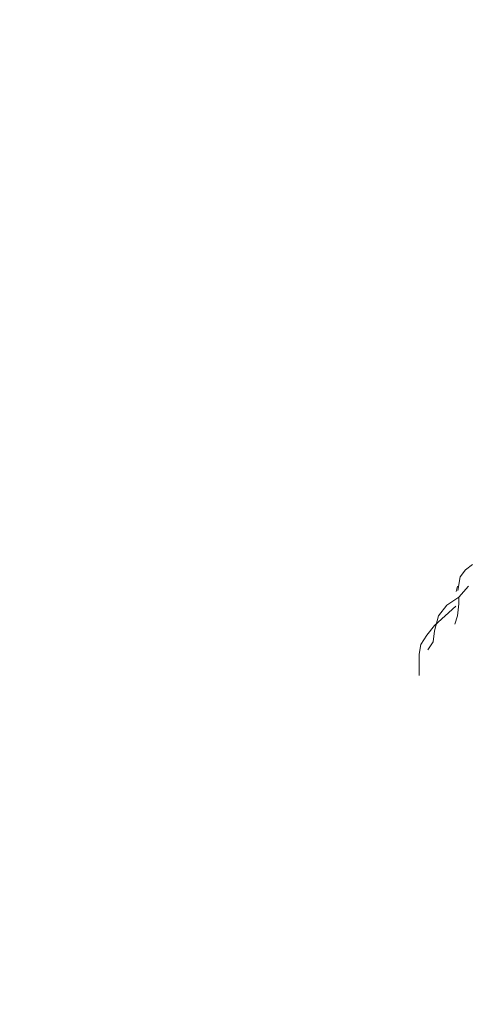
# Model space of a CAD drawing. Units: millimetres. Extents: x 595116 to 630915, y 909473 to 920225.
# Tile 81 of 134: x 629702.75 to 629711.18, y 919266.51 to 919285.1. Entities that reach past the tile are written whole.
import ezdxf

# ---------------------------------------------------------------- set-up
doc = ezdxf.new("R2010")
doc.units = ezdxf.units.MM
doc.layers.add('Dimension', color=3, linetype='Continuous', lineweight=18)
doc.layers.add('L-PLNT', color=85, linetype='Continuous', lineweight=13)
doc.styles.get("Standard").update_dxf_attribs({"font": 'arial.ttf'})
doc.dimstyles.new('ISO-25', dxfattribs={"dimtxt": 9, "dimasz": 6, "dimexe": 1.25, "dimexo": 0.625, "dimtad": 1, "dimlunit": 4, "dimtxsty": 'Standard', "dimcen": 2.5, "dimadec": 0, "dimazin": 0, "dimtfac": 1, "dimtmove": 0, "dimatfit": 3, "dimfxl": 1, "dimarcsym": 0})

# ---------------------------------------------------------------- blocks, each defined once
blk = doc.blocks.new('A$C4FB75ABC')
for p, q in [((0.207, 2.0172), (0.2342, 2.0512)), ((0.2342, 2.0512), (0.2683, 2.0784)), ((0.195, 1.9478), (0.207, 2.0172)), ((0.1865, 1.9422), (0.1934, 1.9695)), ((0.2479, 1.9695), (0.2002, 1.915)), ((0.2002, 1.915), (0.1389, 1.8742)), ((0.2002, 1.915), (0.2002, 1.881)), ((0.1844, 1.8695), (0.0777, 1.7725)), ((0.1389, 1.8742), (0.098, 1.8197)), ((0.2002, 1.881), (0.1934, 1.8197)), ((0.098, 1.8197), (0.0775, 1.7448)), ((0.1934, 1.8197), (0.1797, 1.7788)), ((0.0777, 1.7725), (0.0388, 1.724)), ((0.0775, 1.7448), (0.0707, 1.6903)), ((0.0388, 1.724), (0.0097, 1.6755)), ((0.0707, 1.6903), (0.0435, 1.6494)), ((0.0097, 1.6755), (0, 1.627)), ((0, 1.627), (0, 1.5494)), ((0, 1.5494), (0, 1.5203))]:
    blk.add_line(p, q)
blk = doc.blocks.new('*D216')
at = {"layer": 'Defpoints', "color": 0, "transparency": 16777216}
for p in [(629743.541, 919411.928), (629505.041, 919411.828), (629743.541, 918832.378)]:
    blk.add_point(p, dxfattribs=at)
at = {"layer": 'Dimension', "color": 0, "lineweight": -2, "transparency": 16777216}
for p, q in [((629505.041, 919411.203), (629505.041, 918831.128)), ((629743.541, 919411.303), (629743.541, 918831.128)), ((629511.041, 918832.378), (629737.541, 918832.378))]:
    blk.add_line(p, q, dxfattribs=at)
at = {"layer": 'Dimension', "color": 0, "transparency": 16777216}
for points in [[(629511.041, 918833.378), (629511.041, 918831.378), (629505.041, 918832.378)], [(629737.541, 918833.378), (629737.541, 918831.378), (629743.541, 918832.378)]]:
    blk.add_solid(points, dxfattribs=at)
at = {"layer": 'Dimension', "color": 0, "transparency": 16777216, "insert": (629624.291, 918837.656), "char_height": 9, "attachment_point": 5}
blk.add_mtext('19\'-10 1/2"', dxfattribs=at)

msp = doc.modelspace()

# ---------------------------------------------------------------- block references
at = {"layer": 'L-PLNT', "xscale": 3.753413438031968, "yscale": 3.753413438031968, "zscale": 3.753413438031968}
msp.add_blockref('A$C4FB75ABC', (629710.284, 919267.014), dxfattribs=at)

# ---------------------------------------------------------------- dimensions: what is measured, and where the dimension line sits
at = {"layer": 'Dimension'}
dim = msp.add_linear_dim(base=(629743.541, 918832.378), p1=(629505.041, 919411.828), p2=(629743.541, 919411.928), dimstyle='ISO-25', override={"dimdec": 1, "dimlfac": 1, "dimrnd": 0, "dimzin": 1, "dimdsep": 46, "dimlunit": 4, "dimfrac": 2}, dxfattribs=at)
dim.commit()
dim.dimension.update_dxf_attribs({"geometry": '*D216', "text_midpoint": (629624.291, 918837.656)})

doc.saveas('drawing.dxf')
